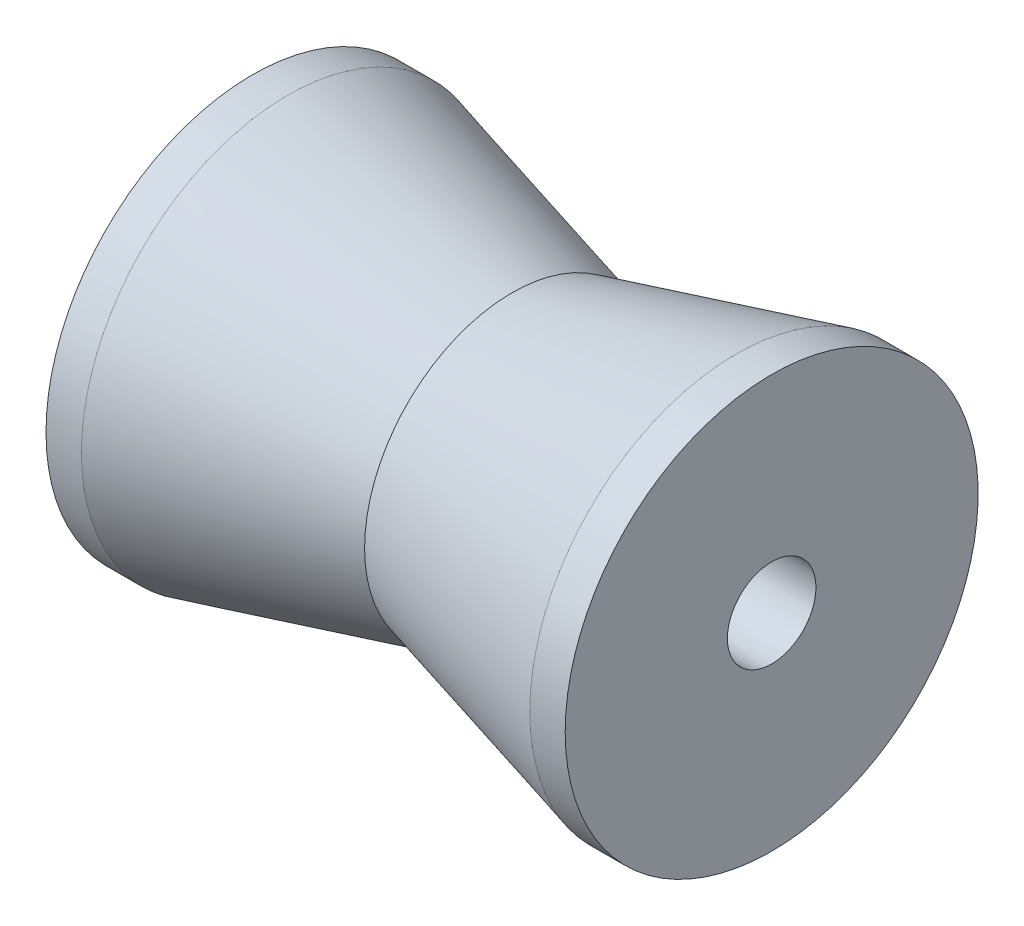
ISO-10303-21;
HEADER;
FILE_DESCRIPTION(('STEP AP214'),'2;1');
FILE_NAME('part.step','',(''),(''),'','','');
FILE_SCHEMA(('AUTOMOTIVE_DESIGN { 1 0 10303 214 1 1 1 1 }'));
ENDSEC;
DATA;
#1=APPLICATION_CONTEXT('core data for automotive mechanical design processes');
#2=APPLICATION_PROTOCOL_DEFINITION('international standard','automotive_design',2000,#1);
#3=PRODUCT_CONTEXT('',#1,'mechanical');
#4=PRODUCT('Part','Part','',(#3));
#5=PRODUCT_RELATED_PRODUCT_CATEGORY('part','',(#4));
#6=PRODUCT_DEFINITION_FORMATION('','',#4);
#7=PRODUCT_DEFINITION_CONTEXT('part definition',#1,'design');
#8=PRODUCT_DEFINITION('design','',#6,#7);
#9=PRODUCT_DEFINITION_SHAPE('','',#8);
#10=(LENGTH_UNIT() NAMED_UNIT(*) SI_UNIT(.MILLI.,.METRE.));
#11=(NAMED_UNIT(*) PLANE_ANGLE_UNIT() SI_UNIT($,.RADIAN.));
#12=(NAMED_UNIT(*) SI_UNIT($,.STERADIAN.) SOLID_ANGLE_UNIT());
#13=UNCERTAINTY_MEASURE_WITH_UNIT(LENGTH_MEASURE(1.E-05),#10,'distance_accuracy_value','');
#14=(GEOMETRIC_REPRESENTATION_CONTEXT(3) GLOBAL_UNCERTAINTY_ASSIGNED_CONTEXT((#13)) GLOBAL_UNIT_ASSIGNED_CONTEXT((#10,
#11,#12)) REPRESENTATION_CONTEXT('',''));
#15=CARTESIAN_POINT('',(0.,0.,0.));
#16=DIRECTION('',(0.,0.,1.));
#17=DIRECTION('',(1.,0.,0.));
#18=AXIS2_PLACEMENT_3D('',#15,#16,#17);
#19=CARTESIAN_POINT('',(38.,25.,0.));
#20=DIRECTION('',(1.,0.,0.));
#21=DIRECTION('',(0.,0.,-1.));
#22=AXIS2_PLACEMENT_3D('',#19,#20,#21);
#23=CONICAL_SURFACE('',#22,35.,0.257323714971089);
#24=CARTESIAN_POINT('',(0.,25.,0.));
#25=DIRECTION('',(-1.,0.,0.));
#26=DIRECTION('',(0.,0.,1.));
#27=AXIS2_PLACEMENT_3D('',#24,#25,#26);
#28=CIRCLE('',#27,25.);
#29=CARTESIAN_POINT('',(0.,25.,25.));
#30=VERTEX_POINT('',#29);
#31=EDGE_CURVE('E65',#30,#30,#28,.T.);
#32=ORIENTED_EDGE('',*,*,#31,.F.);
#33=EDGE_LOOP('',(#32));
#34=FACE_BOUND('',#33,.T.);
#35=CARTESIAN_POINT('',(38.,25.,0.));
#36=DIRECTION('',(-1.,0.,0.));
#37=DIRECTION('',(0.,0.,1.));
#38=AXIS2_PLACEMENT_3D('',#35,#36,#37);
#39=CIRCLE('',#38,35.);
#40=CARTESIAN_POINT('',(38.,25.,35.));
#41=VERTEX_POINT('',#40);
#42=EDGE_CURVE('E10',#41,#41,#39,.T.);
#43=ORIENTED_EDGE('',*,*,#42,.T.);
#44=EDGE_LOOP('',(#43));
#45=FACE_BOUND('',#44,.T.);
#46=ADVANCED_FACE('F40',(#34,#45),#23,.T.);
#47=CARTESIAN_POINT('',(-44.,25.,0.));
#48=DIRECTION('',(-1.,0.,0.));
#49=DIRECTION('',(0.,0.,1.));
#50=AXIS2_PLACEMENT_3D('',#47,#48,#49);
#51=CYLINDRICAL_SURFACE('',#50,35.);
#52=ORIENTED_EDGE('',*,*,#42,.F.);
#53=EDGE_LOOP('',(#52));
#54=FACE_BOUND('',#53,.T.);
#55=CARTESIAN_POINT('',(44.,25.,0.));
#56=DIRECTION('',(-1.,0.,0.));
#57=DIRECTION('',(0.,0.,1.));
#58=AXIS2_PLACEMENT_3D('',#55,#56,#57);
#59=CIRCLE('',#58,35.);
#60=CARTESIAN_POINT('',(44.,25.,35.));
#61=VERTEX_POINT('',#60);
#62=EDGE_CURVE('E43',#61,#61,#59,.T.);
#63=ORIENTED_EDGE('',*,*,#62,.T.);
#64=EDGE_LOOP('',(#63));
#65=FACE_BOUND('',#64,.T.);
#66=ADVANCED_FACE('F66',(#54,#65),#51,.T.);
#67=CARTESIAN_POINT('',(44.,60.,0.));
#68=DIRECTION('',(-1.,0.,0.));
#69=DIRECTION('',(0.,0.,1.));
#70=AXIS2_PLACEMENT_3D('',#67,#68,#69);
#71=PLANE('',#70);
#72=ORIENTED_EDGE('',*,*,#62,.F.);
#73=EDGE_LOOP('',(#72));
#74=FACE_BOUND('',#73,.T.);
#75=CARTESIAN_POINT('',(44.,25.,0.));
#76=DIRECTION('',(-1.,0.,0.));
#77=DIRECTION('',(0.,0.,1.));
#78=AXIS2_PLACEMENT_3D('',#75,#76,#77);
#79=CIRCLE('',#78,7.5);
#80=CARTESIAN_POINT('',(44.,25.,7.5));
#81=VERTEX_POINT('',#80);
#82=EDGE_CURVE('E50',#81,#81,#79,.T.);
#83=ORIENTED_EDGE('',*,*,#82,.T.);
#84=EDGE_LOOP('',(#83));
#85=FACE_BOUND('',#84,.T.);
#86=ADVANCED_FACE('F71',(#74,#85),#71,.F.);
#87=CARTESIAN_POINT('',(-44.,25.,0.));
#88=DIRECTION('',(-1.,0.,0.));
#89=DIRECTION('',(0.,0.,1.));
#90=AXIS2_PLACEMENT_3D('',#87,#88,#89);
#91=CYLINDRICAL_SURFACE('',#90,7.5);
#92=ORIENTED_EDGE('',*,*,#82,.F.);
#93=EDGE_LOOP('',(#92));
#94=FACE_BOUND('',#93,.T.);
#95=CARTESIAN_POINT('',(-44.,25.,0.));
#96=DIRECTION('',(-1.,0.,0.));
#97=DIRECTION('',(0.,0.,1.));
#98=AXIS2_PLACEMENT_3D('',#95,#96,#97);
#99=CIRCLE('',#98,7.5);
#100=CARTESIAN_POINT('',(-44.,25.,7.5));
#101=VERTEX_POINT('',#100);
#102=EDGE_CURVE('E51',#101,#101,#99,.T.);
#103=ORIENTED_EDGE('',*,*,#102,.T.);
#104=EDGE_LOOP('',(#103));
#105=FACE_BOUND('',#104,.T.);
#106=ADVANCED_FACE('F79',(#94,#105),#91,.F.);
#107=CARTESIAN_POINT('',(-44.,60.,0.));
#108=DIRECTION('',(1.,0.,0.));
#109=DIRECTION('',(0.,0.,-1.));
#110=AXIS2_PLACEMENT_3D('',#107,#108,#109);
#111=PLANE('',#110);
#112=ORIENTED_EDGE('',*,*,#102,.F.);
#113=EDGE_LOOP('',(#112));
#114=FACE_BOUND('',#113,.T.);
#115=CARTESIAN_POINT('',(-44.,25.,0.));
#116=DIRECTION('',(-1.,0.,0.));
#117=DIRECTION('',(0.,0.,1.));
#118=AXIS2_PLACEMENT_3D('',#115,#116,#117);
#119=CIRCLE('',#118,35.);
#120=CARTESIAN_POINT('',(-44.,25.,35.));
#121=VERTEX_POINT('',#120);
#122=EDGE_CURVE('E57',#121,#121,#119,.T.);
#123=ORIENTED_EDGE('',*,*,#122,.T.);
#124=EDGE_LOOP('',(#123));
#125=FACE_BOUND('',#124,.T.);
#126=ADVANCED_FACE('F81',(#114,#125),#111,.F.);
#127=CARTESIAN_POINT('',(-44.,25.,0.));
#128=DIRECTION('',(-1.,0.,0.));
#129=DIRECTION('',(0.,0.,1.));
#130=AXIS2_PLACEMENT_3D('',#127,#128,#129);
#131=CYLINDRICAL_SURFACE('',#130,35.);
#132=ORIENTED_EDGE('',*,*,#122,.F.);
#133=EDGE_LOOP('',(#132));
#134=FACE_BOUND('',#133,.T.);
#135=CARTESIAN_POINT('',(-38.,25.,0.));
#136=DIRECTION('',(-1.,0.,0.));
#137=DIRECTION('',(0.,0.,1.));
#138=AXIS2_PLACEMENT_3D('',#135,#136,#137);
#139=CIRCLE('',#138,35.);
#140=CARTESIAN_POINT('',(-38.,25.,35.));
#141=VERTEX_POINT('',#140);
#142=EDGE_CURVE('E56',#141,#141,#139,.T.);
#143=ORIENTED_EDGE('',*,*,#142,.T.);
#144=EDGE_LOOP('',(#143));
#145=FACE_BOUND('',#144,.T.);
#146=ADVANCED_FACE('F86',(#134,#145),#131,.T.);
#147=CARTESIAN_POINT('',(0.,25.,0.));
#148=DIRECTION('',(-1.,0.,0.));
#149=DIRECTION('',(0.,0.,1.));
#150=AXIS2_PLACEMENT_3D('',#147,#148,#149);
#151=CONICAL_SURFACE('',#150,25.,0.257323714971089);
#152=ORIENTED_EDGE('',*,*,#142,.F.);
#153=EDGE_LOOP('',(#152));
#154=FACE_BOUND('',#153,.T.);
#155=ORIENTED_EDGE('',*,*,#31,.T.);
#156=EDGE_LOOP('',(#155));
#157=FACE_BOUND('',#156,.T.);
#158=ADVANCED_FACE('F67',(#154,#157),#151,.T.);
#159=CLOSED_SHELL('',(#46,#66,#86,#106,#126,#146,#158));
#160=MANIFOLD_SOLID_BREP('B2',#159);
#161=ADVANCED_BREP_SHAPE_REPRESENTATION('',(#18,#160),#14);
#162=SHAPE_DEFINITION_REPRESENTATION(#9,#161);
ENDSEC;
END-ISO-10303-21;
